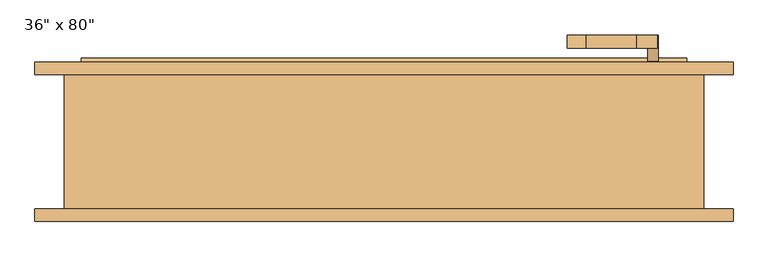
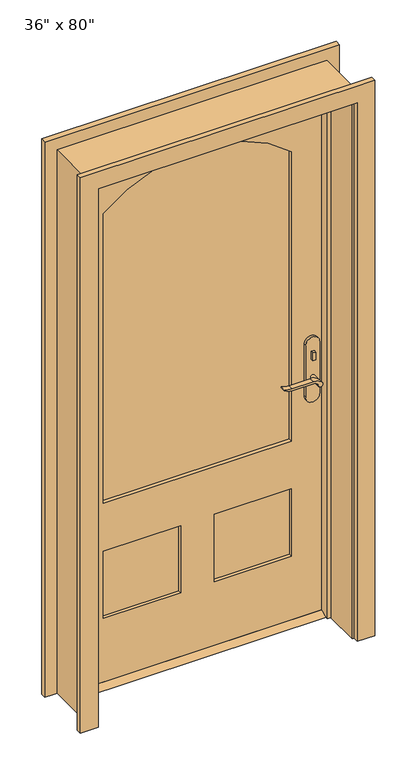
"""IFC4 building model written with IfcOpenShell, lengths in millimetres: door geometry."""

from ifc_helpers import new_model, si_unit, point, frame, frame_2d, origin, place, context, project, spatial, polyline, circle_curve, trimmed, segment, composite_curve, outline, extrude, faceted_brep, source, transform, mapped, element, save


def door_1768e003(model_context):
    return source(origin(), model_context, "Body", "SolidModel", [
        extrude(outline(polyline([(63.5, 12.7), (98.425, 12.7), (123.825, 0.0), (38.1, 0.0), (63.5, 12.7)])), frame((-457.2, 0.0, 0.0), z_axis=(1.0, 0.0, 0.0), x_axis=(0.0, 1.0, 0.0)), (0.0, 0.0, 1.0), 914.4),
        extrude(outline(polyline([(411.4, 43.5), (401.4, 43.5), (401.4, 53.5), (411.4, 53.5), (411.4, 43.5)])), frame((0.0, 0.0, 981.9), z_axis=(0.0, 0.0, 1.0), x_axis=(1.0, 0.0, 0.0)), (0.0, 0.0, 1.0), 30.0),
        extrude(outline(composite_curve([segment(trimmed(circle_curve(frame_2d((996.9, 406.4)), 8.0), [point((996.9, 398.4))], [point((996.9, 414.4))], False, "CARTESIAN"), True, "CONTINUOUS"), segment(trimmed(circle_curve(frame_2d((996.9, 406.4)), 8.0), [point((996.9, 414.4))], [point((996.9, 398.4))], False, "CARTESIAN"), True, "CONTINUOUS")], self_intersect=False)), frame((0.0, 108.425, 0.0), z_axis=(0.0, 1.0, 0.0), x_axis=(0.0, 0.0, 1.0)), (0.0, 0.0, 1.0), 10.0),
        extrude(outline(composite_curve([segment(trimmed(circle_curve(frame_2d((897.1555521, 382.7324871)), 37.2832219), [point((919.0523287, 412.9081363))], [point((934.4, 381.0325667))], False, "CARTESIAN"), True, "CONTINUOUS"), segment(polyline([(934.4, 381.0325667), (934.4, 304.7564091)]), True, "CONTINUOUS"), segment(trimmed(circle_curve(frame_2d((1017.6850638, 304.8227909)), 83.2850902), [point((934.4, 304.7564091))], [point((939.4, 276.4))], True, "CARTESIAN"), True, "CONTINUOUS"), segment(polyline([(939.4, 276.4), (936.6135558, 276.4)]), True, "CONTINUOUS"), segment(trimmed(circle_curve(frame_2d((986.6709207, 308.3396612)), 59.3791355), [point((936.6135558, 276.4))], [point((927.4, 304.7564091))], False, "CARTESIAN"), True, "CONTINUOUS"), segment(polyline([(927.4, 304.7564091), (927.4, 381.0138099)]), True, "CONTINUOUS"), segment(trimmed(circle_curve(frame_2d((909.2738613, 381.0138099)), 18.1261387), [point((927.4, 381.0138099))], [point((914.4, 398.4))], True, "CARTESIAN"), True, "CONTINUOUS"), segment(trimmed(circle_curve(frame_2d((914.4, 406.4)), 8.0), [point((914.4, 398.4))], [point((919.0523287, 412.9081363))], False, "CARTESIAN"), True, "CONTINUOUS")], self_intersect=False)), frame((0.0, 3.5, 0.0), z_axis=(0.0, 1.0, 0.0), x_axis=(0.0, 0.0, 1.0)), (0.0, 0.0, 1.0), 20.0),
        extrude(outline(composite_curve([segment(trimmed(circle_curve(frame_2d((914.4, 406.4)), 8.0), [point((914.3999903, 398.4))], [point((919.0523287, 412.9081363))], False, "CARTESIAN"), True, "CONTINUOUS"), segment(trimmed(circle_curve(frame_2d((897.1555521, 382.7324871)), 37.2832219), [point((919.0523287, 412.9081363))], [point((934.4, 381.0325667))], False, "CARTESIAN"), True, "CONTINUOUS"), segment(polyline([(934.4, 381.0325667), (934.4, 304.7564091)]), True, "CONTINUOUS"), segment(trimmed(circle_curve(frame_2d((1017.6850638, 304.8227909)), 83.2850902), [point((934.4, 304.7564091))], [point((939.4, 276.4))], True, "CARTESIAN"), True, "CONTINUOUS"), segment(polyline([(939.4, 276.4), (936.6135558, 276.4)]), True, "CONTINUOUS"), segment(trimmed(circle_curve(frame_2d((986.6709207, 308.3396612)), 59.3791355), [point((936.6135558, 276.4))], [point((927.4, 304.7564091))], False, "CARTESIAN"), True, "CONTINUOUS"), segment(polyline([(927.4, 304.7564091), (927.4, 381.0138122)]), True, "CONTINUOUS"), segment(trimmed(circle_curve(frame_2d((909.2738682, 381.0138122)), 18.1261318), [point((927.4, 381.0138122))], [point((914.3999903, 398.4))], True, "CARTESIAN"), True, "CONTINUOUS")], self_intersect=False)), frame((0.0, 138.425, 0.0), z_axis=(0.0, 1.0, 0.0), x_axis=(0.0, 0.0, 1.0)), (0.0, 0.0, 1.0), 20.0),
        extrude(outline(composite_curve([segment(trimmed(circle_curve(frame_2d((914.4, 406.4)), 8.0), [point((914.4, 398.4))], [point((914.4, 414.4))], False, "CARTESIAN"), True, "CONTINUOUS"), segment(trimmed(circle_curve(frame_2d((914.4, 406.4)), 8.0), [point((914.4, 414.4))], [point((914.4, 398.4))], False, "CARTESIAN"), True, "CONTINUOUS")], self_intersect=False)), frame((0.0, 23.5, 0.0), z_axis=(0.0, 1.0, 0.0), x_axis=(0.0, 0.0, 1.0)), (0.0, 0.0, 1.0), 30.0),
        extrude(outline(composite_curve([segment(trimmed(circle_curve(frame_2d((914.4, 406.4)), 8.0), [point((914.4, 398.4))], [point((914.4, 414.4))], False, "CARTESIAN"), True, "CONTINUOUS"), segment(trimmed(circle_curve(frame_2d((914.4, 406.4)), 8.0), [point((914.4, 414.4))], [point((914.4, 398.4))], False, "CARTESIAN"), True, "CONTINUOUS")], self_intersect=False)), frame((0.0, 108.425, 0.0), z_axis=(0.0, 1.0, 0.0), x_axis=(0.0, 0.0, 1.0)), (0.0, 0.0, 1.0), 30.0),
        extrude(outline(composite_curve([segment(polyline([(844.4, 431.4), (1039.4, 431.4)]), True, "CONTINUOUS"), segment(trimmed(circle_curve(frame_2d((1039.4, 406.4)), 25.0), [point((1039.4, 431.4))], [point((1039.4, 381.4))], False, "CARTESIAN"), True, "CONTINUOUS"), segment(polyline([(1039.4, 381.4), (844.4, 381.4)]), True, "CONTINUOUS"), segment(trimmed(circle_curve(frame_2d((844.4, 406.4)), 25.0), [point((844.4, 381.4))], [point((844.4, 431.4))], False, "CARTESIAN"), True, "CONTINUOUS")], self_intersect=False)), frame((0.0, 53.5, 0.0), z_axis=(0.0, 1.0, 0.0), x_axis=(0.0, 0.0, 1.0)), (0.0, 0.0, 1.0), 10.0),
        extrude(outline(composite_curve([segment(polyline([(844.4, 431.4), (1039.4, 431.4)]), True, "CONTINUOUS"), segment(trimmed(circle_curve(frame_2d((1039.4, 406.4)), 25.0), [point((1039.4, 431.4))], [point((1039.4, 381.4))], False, "CARTESIAN"), True, "CONTINUOUS"), segment(polyline([(1039.4, 381.4), (844.4, 381.4)]), True, "CONTINUOUS"), segment(trimmed(circle_curve(frame_2d((844.4, 406.4)), 25.0), [point((844.4, 381.4))], [point((844.4, 431.4))], False, "CARTESIAN"), True, "CONTINUOUS")], self_intersect=False)), frame((0.0, 98.425, 0.0), z_axis=(0.0, 1.0, 0.0), x_axis=(0.0, 0.0, 1.0)), (0.0, 0.0, 1.0), 10.0),
        extrude(outline(polyline([(2032.0, -457.2), (12.7, -457.2), (12.7, 457.2), (2032.0, 457.2), (2032.0, -457.2)]), holes=[composite_curve([segment(polyline([(688.975, -336.55), (1784.35, -336.55)]), True, "CONTINUOUS"), segment(trimmed(circle_curve(frame_2d((1401.92125, 0.0)), 509.42875), [point((1784.35, -336.55))], [point((1784.35, 336.55))], True, "CARTESIAN"), True, "CONTINUOUS"), segment(polyline([(1784.35, 336.55), (688.975, 336.55), (688.975, -336.55)]), True, "CONTINUOUS")], self_intersect=False), polyline([(508.0, -60.325), (254.0, -60.325), (254.0, -336.55), (508.0, -336.55), (508.0, -60.325)]), polyline([(508.0, 336.55), (254.0, 336.55), (254.0, 60.325), (508.0, 60.325), (508.0, 336.55)])]), frame((0.0, 63.5, 0.0), z_axis=(0.0, 1.0, 0.0), x_axis=(0.0, 0.0, 1.0)), (0.0, 0.0, 1.0), 34.925),
        faceted_brep([(482.6, 98.425, 0.0), (482.6, -104.775, 0.0), (457.2, -104.775, 0.0), (457.2, 28.575, 0.0), (444.5, 28.575, 0.0), (444.5, 63.5, 0.0), (457.2, 63.5, 0.0), (457.2, 98.425, 0.0), (482.6, 98.425, 2057.4), (482.6, -104.775, 2057.4), (-482.6, -104.775, 2057.4), (-482.6, -104.775, 0.0), (-457.2, -104.775, 0.0), (-457.2, -104.775, 2032.0), (457.2, -104.775, 2032.0), (457.2, 28.575, 2032.0), (-457.2, 28.575, 2032.0), (-457.2, 28.575, 0.0), (-444.5, 28.575, 0.0), (-444.5, 28.575, 2019.3), (444.5, 28.575, 2019.3), (444.5, 63.5, 2019.3), (-444.5, 63.5, 2019.3), (-444.5, 63.5, 0.0), (-457.2, 63.5, 0.0), (-457.2, 63.5, 2032.0), (457.2, 63.5, 2032.0), (457.2, 98.425, 2032.0), (-457.2, 98.425, 2032.0), (-457.2, 98.425, 0.0), (-482.6, 98.425, 0.0), (-482.6, 98.425, 2057.4)], [[[0, 1, 2, 3, 4, 5, 6, 7]], [[1, 0, 8, 9]], [[2, 1, 9, 10, 11, 12, 13, 14]], [[3, 2, 14, 15]], [[4, 3, 15, 16, 17, 18, 19, 20]], [[5, 4, 20, 21]], [[6, 5, 21, 22, 23, 24, 25, 26]], [[7, 6, 26, 27]], [[0, 7, 27, 28, 29, 30, 31, 8]], [[9, 8, 31, 10]], [[15, 14, 13, 16]], [[21, 20, 19, 22]], [[27, 26, 25, 28]], [[30, 29, 24, 23, 18, 17, 12, 11]], [[10, 31, 30, 11]], [[16, 13, 12, 17]], [[22, 19, 18, 23]], [[28, 25, 24, 29]]]),
        extrude(outline(polyline([(-60.325, 75.1416667), (-336.55, 75.1416667), (-336.55, 86.7833333), (-60.325, 86.7833333), (-60.325, 75.1416667)])), frame((0.0, 0.0, 254.0), z_axis=(0.0, 0.0, 1.0), x_axis=(1.0, 0.0, 0.0)), (0.0, 0.0, 1.0), 254.0),
        extrude(outline(polyline([(336.55, 75.1416667), (60.325, 75.1416667), (60.325, 86.7833333), (336.55, 86.7833333), (336.55, 75.1416667)])), frame((0.0, 0.0, 254.0), z_axis=(0.0, 0.0, 1.0), x_axis=(1.0, 0.0, 0.0)), (0.0, 0.0, 1.0), 254.0),
        extrude(outline(composite_curve([segment(polyline([(688.975, -336.55), (688.975, 336.55), (1784.35, 336.55)]), True, "CONTINUOUS"), segment(trimmed(circle_curve(frame_2d((1401.92125, 0.0)), 509.42875), [point((1784.35, 336.55))], [point((1784.35, -336.55))], False, "CARTESIAN"), True, "CONTINUOUS"), segment(polyline([(1784.35, -336.55), (688.975, -336.55)]), True, "CONTINUOUS")], self_intersect=False)), frame((0.0, 77.47, 0.0), z_axis=(0.0, 1.0, 0.0), x_axis=(0.0, 0.0, 1.0)), (0.0, 0.0, 1.0), 6.985),
        extrude(outline(polyline([(0.0, -527.05), (0.0, -463.55), (2038.35, -463.55), (2038.35, 463.55), (0.0, 463.55), (0.0, 527.05), (2101.85, 527.05), (2101.85, -527.05), (0.0, -527.05)])), frame((0.0, -123.825, 0.0), z_axis=(0.0, 1.0, 0.0), x_axis=(0.0, 0.0, 1.0)), (0.0, 0.0, 1.0), 19.05),
        extrude(outline(polyline([(0.0, -527.05), (0.0, -463.55), (2038.35, -463.55), (2038.35, 463.55), (0.0, 463.55), (0.0, 527.05), (2101.85, 527.05), (2101.85, -527.05), (0.0, -527.05)])), frame((0.0, 98.425, 0.0), z_axis=(0.0, 1.0, 0.0), x_axis=(0.0, 0.0, 1.0)), (0.0, 0.0, 1.0), 19.05),
    ])


if __name__ == "__main__":
    model = new_model("IFC4")
    model_context = context("Model", 3, world=origin())
    ifc_project = project(units=[si_unit("LENGTHUNIT", "METRE", prefix="MILLI")], contexts=[model_context])
    site = spatial("IfcSite", under=ifc_project)
    building = spatial("IfcBuilding", under=site)
    placement = place(None, origin())
    door_shape = door_1768e003(model_context)
    element("IfcDoor", 1, ObjectType="36\" x 80\"", at=placement, inside=building, context=model_context, shape_type="MappedRepresentation", body=[
        mapped(door_shape, transform((0.0, 0.0, 0.0), x_axis=(1.0, 0.0, 0.0), y_axis=(0.0, 1.0, 0.0), z_axis=(0.0, 0.0, 1.0))),
    ])
    save(model, "model.ifc")

# Revit data of these elements
# Type "36\" x 80\""
#   Type Mark = "11"
#   Assembly Code = "B2030100"
#   Analytic Construction = "French door, wood frame with single glass"
#   Threshold Offset [instance default] = 0' - 0 1/2"
#   Thickness = 0' - 1 3/8"
#   Thermal Resistance (R) = 1.0696 (h·ft²·°F)/BTU
#   Swing Angle [instance default] = 90.00°
#   Stiles = 0' - 4 3/4"
#   Rough Width = 3' - 2"
#   Rough Height = 6' - 9"
#   Radius = 1' - 8.05625"
#   Lock Rail = 0' - 7 1/8"
#   Height = 6' - 8"
#   Width = 3' - 0"
#   Heat Transfer Coefficient (U) = 0.9350 BTU/(h·ft²·°F)
#   Door Offset [instance default] = 0' - 0"
#   Bottom Rail = 0' - 9 1/2"
#   Threshold [instance default] = yes
#   Function = 1
#   Exterior Trim [instance default] = yes
#   Trim Material = Cherry
#   Threshold Material = Cherry
#   Panel Material = Cherry
#   Glazing = Glass
#   Frame Material = Cherry
#   Door Handle Material = Aluminum
#   Visual Light Transmittance = 0
#   Solar Heat Gain Coefficient = 0
#   Wall Closure = (empty or 0)
#   Construction Type = (empty or 0)
# Element 1 (IfcDoor, "36\" x 80\"")
#   Materials on its faces: "Cherry", "Aluminum", "Glass"
# Materials
#   "Cherry": class "Wood", colour RGB 226 177 128, transparency 0, Description = "Prunus Serotina", Cost = 0
#   "Glass": class "Glass", colour RGB 0 128 192, transparency 0.75, Description = "Soda Lime Glass", Cost = 0
#   "Aluminum": class "Metal", colour RGB 247 247 247, transparency 0, Description = "Aluminum 6061", Cost = 0
